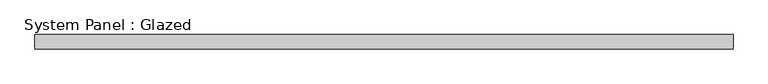
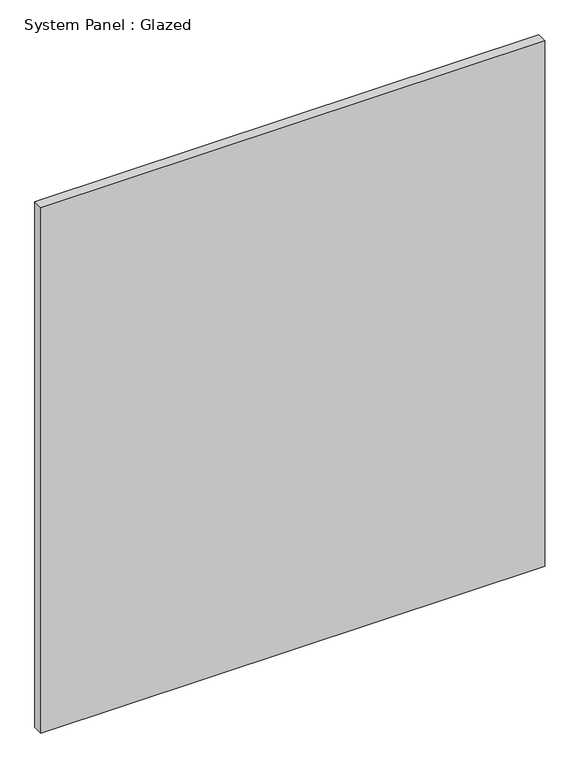
"""IFC4 building model written with IfcOpenShell, lengths in millimetres: plate geometry, System Panel : Glazed."""

from ifc_helpers import new_model, si_unit, origin, origin_with_axes, place, context, project, spatial, polyline, outline, extrude, source, transform, mapped, element, save


def system_panel_glazed_b055ca82(model_context):
    return source(origin(), model_context, "Body", "SweptSolid", [
        extrude(outline(polyline([(603.3504479, 24.5), (-603.3504479, 24.5), (-603.3504479, 49.5), (603.3504479, 49.5), (603.3504479, 24.5)])), origin_with_axes(), (0.0, 0.0, 1.0), 1330.8429687),
    ])


if __name__ == "__main__":
    model = new_model("IFC4")
    model_context = context("Model", 3, world=origin())
    ifc_project = project(units=[si_unit("LENGTHUNIT", "METRE", prefix="MILLI")], contexts=[model_context])
    site = spatial("IfcSite", under=ifc_project)
    building = spatial("IfcBuilding", under=site)
    placement = place(None, origin())
    system_panel_glazed_shape = system_panel_glazed_b055ca82(model_context)
    element("IfcPlate", 1, ObjectType="System Panel : Glazed", at=placement, inside=building, context=model_context, shape_type="MappedRepresentation", body=[
        mapped(system_panel_glazed_shape, transform((0.0, 0.0, 0.0), x_axis=(1.0, 0.0, 0.0), y_axis=(0.0, 1.0, 0.0), z_axis=(0.0, 0.0, 1.0))),
    ])
    save(model, "model.ifc")

# Revit data of these elements
# Type "System Panel : Glazed"
#   Keynote = "H11"
#   Construction Type Id = "GSP4R"
#   Analytic Construction = "1/8 in Pilkington single glazing"
#   Visual Light Transmittance = 0.9
#   Solar Heat Gain Coefficient = 0.86
#   Heat Transfer Coefficient (U) = 6.7069 W/(m²·K)
#   Define Thermal Properties by = 1
# Element 1 (IfcPlate, "System Panel : Glazed")
#   Materials on its faces: "Glass"
# Materials
#   "Glass": class "Glass", colour RGB 0 128 192, transparency 0.9, Description = "Soda Lime Glass", Cost = 0
